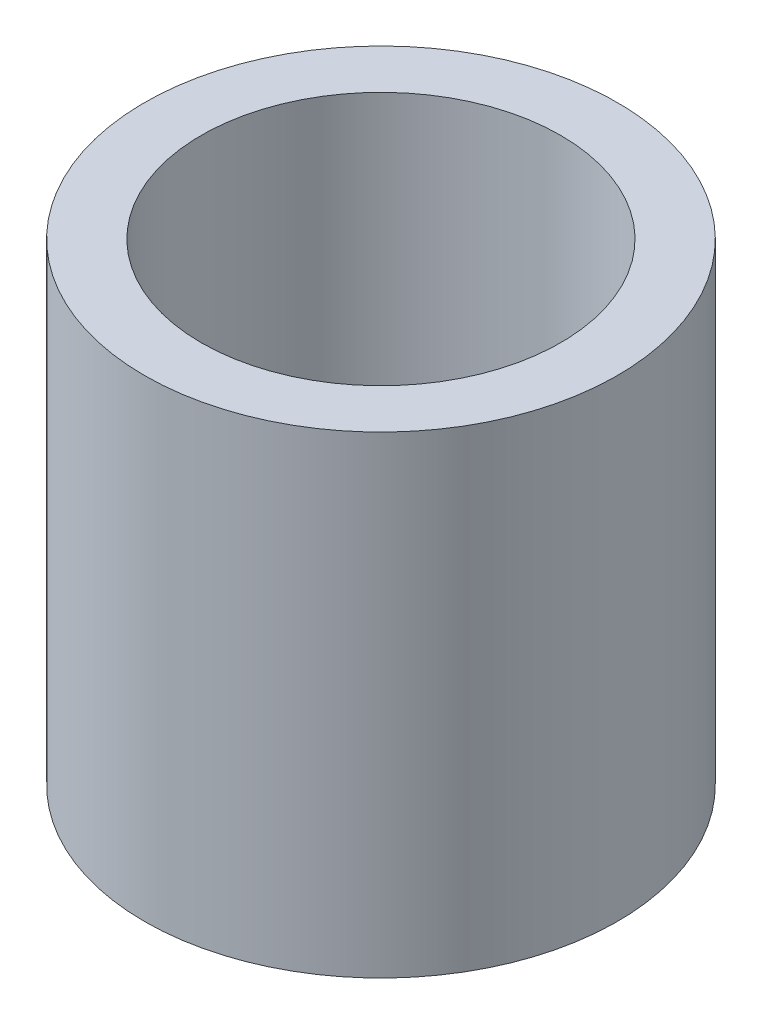
from build123d import *

# Parameters (mm, degrees)
BUSHING_PROFILE_25X_19_R   = 12.5
BUSHING_PROFILE_25X_19_R_2 = 9.5
BUSHING_BODY_L25_DEPTH     = 25


with BuildPart() as part:
    # Bushing Profile Ø25xØ19 → Bushing Body L25 (new body)
    with BuildSketch(Plane(origin=(0, 0, 0), x_dir=(1, 0, 0), z_dir=(0, 1, 0))):
        with Locations(Location((0, 0, 0), (0, 0, 270))):
            Circle(BUSHING_PROFILE_25X_19_R)
        with Locations(Location((0, 0, 0), (0, 0, 270))):
            Circle(BUSHING_PROFILE_25X_19_R_2, mode=Mode.SUBTRACT)
    extrude(amount=BUSHING_BODY_L25_DEPTH)


solid = part.part
